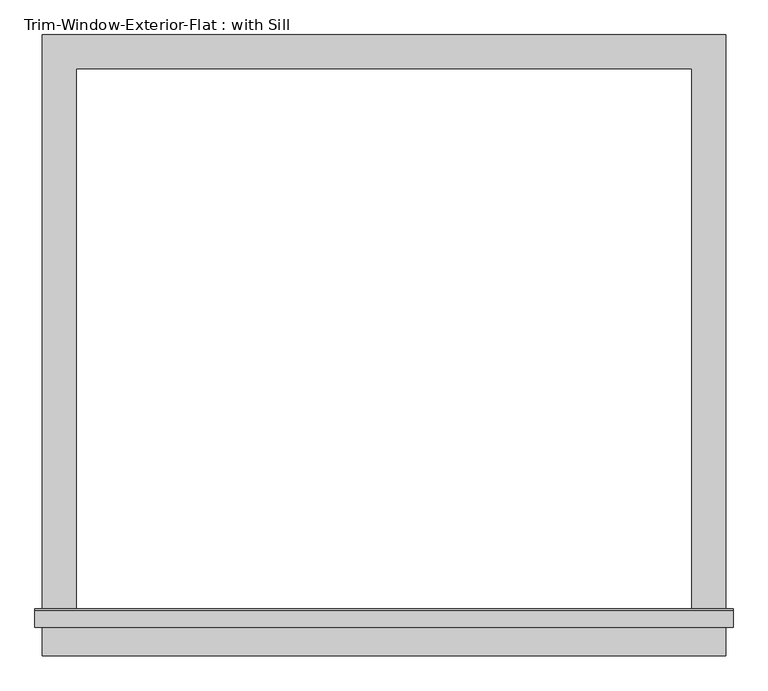
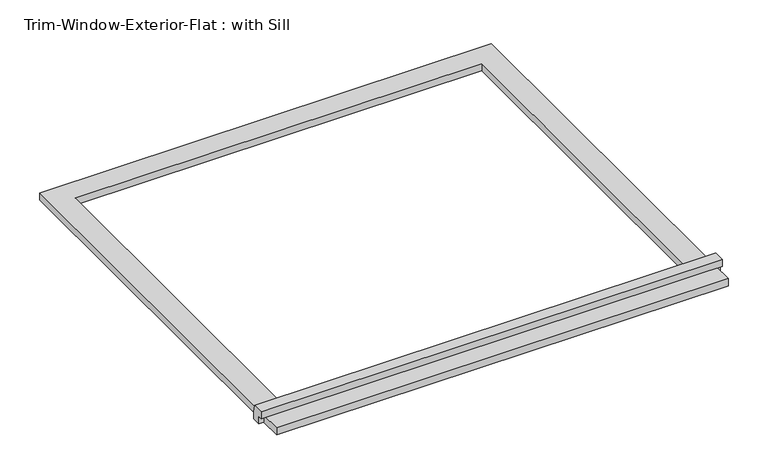
"""IFC4 building model written with IfcOpenShell, lengths in millimetres: proxy geometry, Trim-Window-Exterior-Flat : with Sill."""

from ifc_helpers import new_model, si_unit, frame, origin, origin_with_axes, place, context, project, spatial, polyline, outline, extrude, source, transform, mapped, element, save


def trim_window_exterior_flat_with_sill_79aa6636(model_context):
    return source(origin(), model_context, "Body", "SweptSolid", [
        extrude(outline(polyline([(577.85, -936.5823709), (577.85, -993.7323709), (-577.85, -993.7323709), (-577.85, -936.5823709), (577.85, -936.5823709)])), origin_with_axes(), (0.0, 0.0, 1.0), 19.05),
        extrude(outline(polyline([(-946.15, 38.1), (-916.8580645, 38.1), (-914.4, 19.05), (-914.4, 0.0), (-936.5823709, 0.0), (-936.5823709, 19.05), (-946.15, 19.05), (-946.15, 38.1)])), frame((-590.55, 0.0, 0.0), z_axis=(1.0, 0.0, 0.0), x_axis=(0.0, 1.0, 0.0)), (0.0, 0.0, 1.0), 1181.1),
        extrude(outline(polyline([(-577.85, 57.15), (577.85, 57.15), (577.85, -914.4), (520.7, -914.4), (520.7, 0.0), (-520.7, 0.0), (-520.7, -914.4), (-577.85, -914.4), (-577.85, 57.15)])), origin_with_axes(), (0.0, 0.0, 1.0), 19.05),
    ])


if __name__ == "__main__":
    model = new_model("IFC4")
    model_context = context("Model", 3, world=origin())
    ifc_project = project(units=[si_unit("LENGTHUNIT", "METRE", prefix="MILLI")], contexts=[model_context])
    site = spatial("IfcSite", under=ifc_project)
    building = spatial("IfcBuilding", under=site)
    placement = place(None, origin())
    trim_window_exterior_flat_with_sill_shape = trim_window_exterior_flat_with_sill_79aa6636(model_context)
    element("IfcBuildingElementProxy", 1, Name="Trim-Window-Exterior-Flat : with Sill", ObjectType="Trim-Window-Exterior-Flat : with Sill", at=placement, inside=building, context=model_context, shape_type="MappedRepresentation", body=[
        mapped(trim_window_exterior_flat_with_sill_shape, transform((0.0, 0.0, 0.0), x_axis=(1.0, 0.0, 0.0), y_axis=(0.0, 1.0, 0.0), z_axis=(0.0, 0.0, 1.0))),
    ])
    save(model, "model.ifc")

# Revit data of these elements
# Type "Trim-Window-Exterior-Flat : with Sill"
#   Trim Width = 0' - 2 1/4"
#   Trim Thickness_Picture Frame = 0' - 1 1/4"
#   Trim Thickness_with Sill = 0' - 0 3/4"
#   Sill Thickness = 0' - 1 1/4"
#   Opening Width [instance default] = 2' - 0"
#   Opening Height [instance default] = 3' - 0"
#   Default Elevation = 4' - 0"
#   Sill = yes
#   Picture Frame = no
#   Trim Material [instance default] = none
# Element 1 (IfcBuildingElementProxy, "Trim-Window-Exterior-Flat : with Sill")
#   Opening Width = 3' - 5"
#   Trim Material = Clad - White
#   Materials on its faces: "Clad - White"
# Materials
#   "Clad - White": class "Wood", colour RGB 242 242 238, transparency 0, Cost = 0
